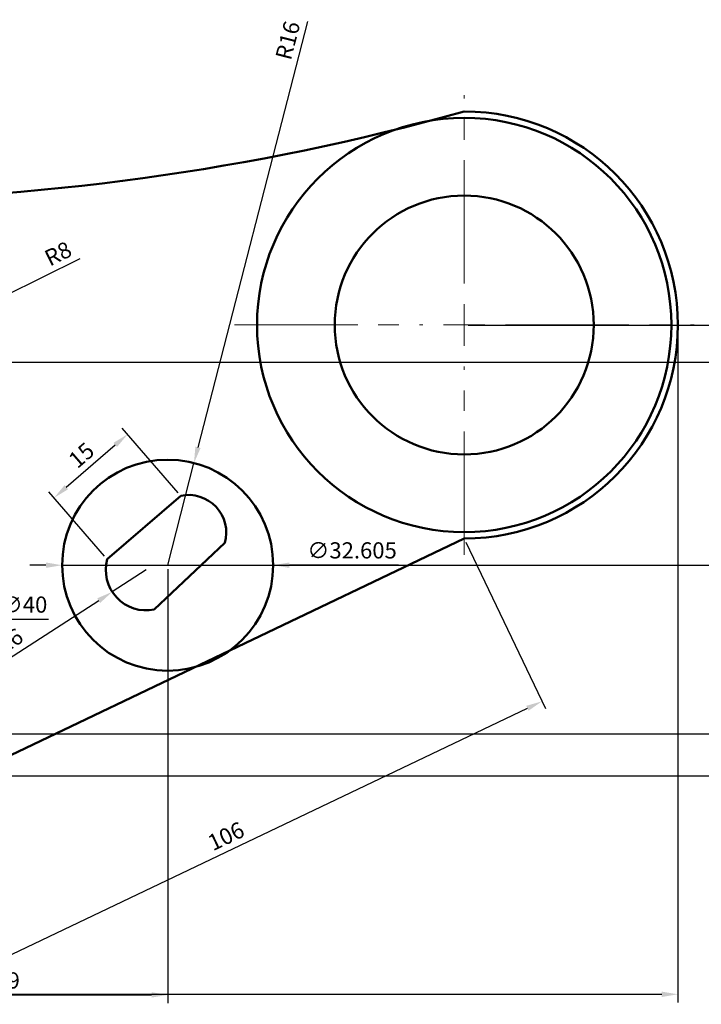
# Model space of a CAD drawing. Units: millimetres. Extents: x 1605 to 2079, y 1280 to 1879.
# Tile 5 of 7: x 1815 to 1920, y 1384 to 1536. Entities that reach past the tile are written whole.
import ezdxf

# ---------------------------------------------------------------- set-up
doc = ezdxf.new("R2010")
doc.units = ezdxf.units.MM
doc.linetypes.add('CENTER2', pattern=[28.575, 19.05, -3.175, 3.175, -3.175])
for name, color, linetype, lineweight in [('M-CNTR', 1, 'CENTER2', 18), ('M-DIMS', 2, 'Continuous', 25), ('M-OUTL', 7, 'Continuous', 50)]:
    doc.layers.add(name, color=color, linetype=linetype, lineweight=lineweight)
doc.styles.get("Standard").update_dxf_attribs({"font": 'arial.ttf'})
doc.dimstyles.new('ISO-25', dxfattribs={"dimtxt": 2.5, "dimasz": 2.5, "dimexe": 1.25, "dimexo": 0.625, "dimtad": 1, "dimdec": 0, "dimtxsty": 'Standard', "dimcen": 2.5, "dimadec": 0, "dimazin": 0, "dimtfac": 1, "dimtdec": 0, "dimtmove": 0, "dimatfit": 3, "dimfxl": 1, "dimarcsym": 0})

# ---------------------------------------------------------------- blocks, each defined once
blk = doc.blocks.new('*U3')
at = {"layer": 'M-CNTR', "color": 0, "transparency": 16777216}
for p, q in [((0, 6.4), (0, 35.5)), ((-35.5, 0), (-6.4, 0)), ((6.4, 0), (35.5, 0)), ((0, -35.5), (0, -6.4))]:
    blk.add_line(p, q, dxfattribs=at)
at = {"layer": 'M-CNTR', "color": 0, "linetype": 'Continuous', "transparency": 16777216}
for p, q in [((0, -3.2), (0, 3.2)), ((-3.2, 0), (3.2, 0))]:
    blk.add_line(p, q, dxfattribs=at)
blk = doc.blocks.new('*D12')
at = {"layer": 'Defpoints', "color": 0, "transparency": 16777216}
for p in [(1650.42, 1488.98), (1916.42, 1488.98), (1916.42, 1385.56)]:
    blk.add_point(p, dxfattribs=at)
at = {"layer": 'M-DIMS', "color": 0, "lineweight": -2, "transparency": 16777216}
for p, q in [((1650.42, 1488.36), (1650.42, 1384.31)), ((1916.42, 1488.36), (1916.42, 1384.31)), ((1652.92, 1385.56), (1913.92, 1385.56))]:
    blk.add_line(p, q, dxfattribs=at)
at = {"layer": 'M-DIMS', "color": 0, "transparency": 16777216}
for points in [[(1652.92, 1385.97), (1652.92, 1385.14), (1650.42, 1385.56)], [(1913.92, 1385.97), (1913.92, 1385.14), (1916.42, 1385.56)]]:
    blk.add_solid(points, dxfattribs=at)
at = {"layer": 'M-DIMS', "color": 0, "transparency": 16777216, "insert": (1783.42, 1387.46), "char_height": 2.5, "attachment_point": 5}
blk.add_mtext('266', dxfattribs=at)
blk = doc.blocks.new('*D18')
at = {"layer": 'Defpoints', "color": 0, "transparency": 16777216}
for p in [(1841.67, 1467.65), (1837.61, 1451.86)]:
    blk.add_point(p, dxfattribs=at)
at = {"layer": 'M-DIMS', "color": 0, "lineweight": -2, "transparency": 16777216}
for p, q in [((1859.21, 1535.89), (1842.29, 1470.07)), ((1837.61, 1451.86), (1841.67, 1467.65))]:
    blk.add_line(p, q, dxfattribs=at)
at = {"layer": 'M-DIMS', "color": 0, "transparency": 16777216}
blk.add_solid([(1841.89, 1470.18), (1842.69, 1469.97), (1841.67, 1467.65)], dxfattribs=at)
at = {"layer": 'M-DIMS', "color": 0, "transparency": 16777216, "insert": (1856.47, 1532.87), "char_height": 2.5, "attachment_point": 5, "rotation": 75.5801}
blk.add_mtext('R16', dxfattribs=at)
blk = doc.blocks.new('*D22')
at = {"layer": 'Defpoints', "color": 0, "transparency": 16777216}
for p in [(1810.14, 1492.31), (1803.42, 1488.98)]:
    blk.add_point(p, dxfattribs=at)
at = {"layer": 'M-DIMS', "color": 0, "lineweight": -2, "transparency": 16777216}
for p, q in [((1824.04, 1499.19), (1812.38, 1493.42)), ((1803.42, 1488.98), (1810.14, 1492.31))]:
    blk.add_line(p, q, dxfattribs=at)
at = {"layer": 'M-DIMS', "color": 0, "transparency": 16777216}
blk.add_solid([(1812.19, 1493.79), (1812.56, 1493.05), (1810.14, 1492.31)], dxfattribs=at)
at = {"layer": 'M-DIMS', "color": 0, "transparency": 16777216, "insert": (1820.82, 1499.72), "char_height": 2.5, "attachment_point": 5, "rotation": 26.3503}
blk.add_mtext('R8', dxfattribs=at)
blk = doc.blocks.new('*D25')
at = {"layer": 'Defpoints', "color": 0, "transparency": 16777216}
for p in [(1883.42, 1455.98), (1895.43, 1430.83), (1787.72, 1410.29)]:
    blk.add_point(p, dxfattribs=at)
at = {"layer": 'M-DIMS', "color": 0, "lineweight": -2, "transparency": 16777216}
for p, q in [((1883.69, 1455.42), (1895.96, 1429.7)), ((1801.99, 1386.22), (1893.17, 1429.75)), ((1787.99, 1409.73), (1800.27, 1384.01))]:
    blk.add_line(p, q, dxfattribs=at)
at = {"layer": 'M-DIMS', "color": 0, "transparency": 16777216}
for points in [[(1892.99, 1430.13), (1893.35, 1429.38), (1895.43, 1430.83)], [(1801.81, 1386.59), (1802.17, 1385.84), (1799.73, 1385.14)]]:
    blk.add_solid(points, dxfattribs=at)
at = {"layer": 'M-DIMS', "color": 0, "transparency": 16777216, "insert": (1846.76, 1409.7), "char_height": 2.5, "attachment_point": 5, "rotation": 25.5234}
blk.add_mtext('106', dxfattribs=at)
blk = doc.blocks.new('*D28')
at = {"layer": 'Defpoints', "color": 0, "transparency": 16777216}
for p in [(1834.3, 1451.14), (1829.05, 1447.75)]:
    blk.add_point(p, dxfattribs=at)
at = {"layer": 'M-DIMS', "color": 0, "lineweight": -2, "transparency": 16777216}
for p, q in [((1834.3, 1451.14), (1829.05, 1447.75)), ((1812.16, 1436.85), (1826.95, 1446.39))]:
    blk.add_line(p, q, dxfattribs=at)
at = {"layer": 'M-DIMS', "color": 0, "transparency": 16777216}
blk.add_solid([(1826.72, 1446.74), (1827.18, 1446.04), (1829.05, 1447.75)], dxfattribs=at)
at = {"layer": 'M-DIMS', "color": 0, "transparency": 16777216, "insert": (1813.35, 1439.88), "char_height": 2.5, "attachment_point": 5, "rotation": 32.8205}
blk.add_mtext('R6', dxfattribs=at)
blk = doc.blocks.new('*D29')
at = {"layer": 'Defpoints', "color": 0, "transparency": 16777216}
for p in [(1831.41, 1472.09), (1839.62, 1462.6), (1828.28, 1452.79)]:
    blk.add_point(p, dxfattribs=at)
at = {"layer": 'M-DIMS', "color": 0, "lineweight": -2, "transparency": 16777216}
for p, q in [((1839.21, 1463.07), (1830.59, 1473.04)), ((1821.95, 1463.91), (1829.51, 1470.45)), ((1827.87, 1453.26), (1819.25, 1463.22))]:
    blk.add_line(p, q, dxfattribs=at)
at = {"layer": 'M-DIMS', "color": 0, "transparency": 16777216}
for points in [[(1829.24, 1470.77), (1829.79, 1470.14), (1831.41, 1472.09)], [(1821.68, 1464.23), (1822.23, 1463.6), (1820.06, 1462.27)]]:
    blk.add_solid(points, dxfattribs=at)
at = {"layer": 'M-DIMS', "color": 0, "transparency": 16777216, "insert": (1824.49, 1468.62), "char_height": 2.5, "attachment_point": 5, "rotation": 40.8746}
blk.add_mtext('15', dxfattribs=at)
blk = doc.blocks.new('*D40')
at = {"layer": 'Defpoints', "color": 0, "transparency": 16777216}
for p in [(1916.42, 1488.98), (1783.42, 1419.31), (2077.9, 1419.31)]:
    blk.add_point(p, dxfattribs=at)
at = {"layer": 'M-DIMS', "color": 0, "lineweight": -2, "transparency": 16777216}
for p, q in [((1917.04, 1488.98), (2079.15, 1488.98)), ((2077.9, 1486.48), (2077.9, 1421.81)), ((1784.04, 1419.31), (2079.15, 1419.31))]:
    blk.add_line(p, q, dxfattribs=at)
at = {"layer": 'M-DIMS', "color": 0, "transparency": 16777216}
for points in [[(2077.48, 1486.48), (2078.32, 1486.48), (2077.9, 1488.98)], [(2077.48, 1421.81), (2078.32, 1421.81), (2077.9, 1419.31)]]:
    blk.add_solid(points, dxfattribs=at)
at = {"layer": 'M-DIMS', "color": 0, "transparency": 16777216, "insert": (2076, 1454.15), "char_height": 2.5, "attachment_point": 5, "rotation": 90}
blk.add_mtext('69.67', dxfattribs=at)
blk = doc.blocks.new('*D43')
at = {"layer": 'Defpoints', "color": 0, "transparency": 16777216}
for p in [(1837.61, 1451.86), (1783.42, 1443.48), (1837.61, 1385.46)]:
    blk.add_point(p, dxfattribs=at)
at = {"layer": 'M-DIMS', "color": 0, "lineweight": -2, "transparency": 16777216}
for p, q in [((1837.61, 1451.24), (1837.61, 1384.21)), ((1783.42, 1442.85), (1783.42, 1384.21)), ((1785.92, 1385.46), (1835.11, 1385.46))]:
    blk.add_line(p, q, dxfattribs=at)
at = {"layer": 'M-DIMS', "color": 0, "transparency": 16777216}
for points in [[(1785.92, 1385.88), (1785.92, 1385.05), (1783.42, 1385.46)], [(1835.11, 1385.88), (1835.11, 1385.05), (1837.61, 1385.46)]]:
    blk.add_solid(points, dxfattribs=at)
at = {"layer": 'M-DIMS', "color": 0, "transparency": 16777216, "insert": (1810.51, 1387.37), "char_height": 2.5, "attachment_point": 5}
blk.add_mtext('54.19', dxfattribs=at)
blk = doc.blocks.new('*D46')
at = {"layer": 'Defpoints', "color": 0, "transparency": 16777216}
for p in [(1883.42, 1488.98), (2077.9, 1488.98), (1837.61, 1451.86)]:
    blk.add_point(p, dxfattribs=at)
at = {"layer": 'M-DIMS', "color": 0, "lineweight": -2, "transparency": 16777216}
for p, q in [((1884.04, 1488.98), (2079.15, 1488.98)), ((2077.9, 1454.36), (2077.9, 1486.48)), ((1838.23, 1451.86), (2079.15, 1451.86))]:
    blk.add_line(p, q, dxfattribs=at)
at = {"layer": 'M-DIMS', "color": 0, "transparency": 16777216}
for points in [[(2077.48, 1486.48), (2078.32, 1486.48), (2077.9, 1488.98)], [(2077.48, 1454.36), (2078.32, 1454.36), (2077.9, 1451.86)]]:
    blk.add_solid(points, dxfattribs=at)
at = {"layer": 'M-DIMS', "color": 0, "transparency": 16777216, "insert": (2076, 1470.42), "char_height": 2.5, "attachment_point": 5, "rotation": 90}
blk.add_mtext('37.12', dxfattribs=at)
blk = doc.blocks.new('*D51')
at = {"layer": 'Defpoints', "color": 0, "transparency": 16777216}
for p in [(1624.07, 1483.2), (1984.76, 1483.2), (1947.57, 1425.73)]:
    blk.add_point(p, dxfattribs=at)
at = {"layer": 'M-DIMS', "color": 0, "lineweight": -2, "transparency": 16777216}
for p, q in [((1984.13, 1483.2), (1622.82, 1483.2)), ((1624.07, 1428.23), (1624.07, 1480.7)), ((1946.94, 1425.73), (1622.82, 1425.73))]:
    blk.add_line(p, q, dxfattribs=at)
at = {"layer": 'M-DIMS', "color": 0, "transparency": 16777216}
for points in [[(1623.65, 1480.7), (1624.48, 1480.7), (1624.07, 1483.2)], [(1623.65, 1428.23), (1624.48, 1428.23), (1624.07, 1425.73)]]:
    blk.add_solid(points, dxfattribs=at)
at = {"layer": 'M-DIMS', "color": 0, "transparency": 16777216, "insert": (1622.17, 1454.47), "char_height": 2.5, "attachment_point": 5, "rotation": 90}
blk.add_mtext('57.47', dxfattribs=at)
blk = doc.blocks.new('*D64')
at = {"layer": 'Defpoints', "color": 0, "transparency": 16777216}
for p in [(1763.42, 1443.48), (1803.42, 1443.48)]:
    blk.add_point(p, dxfattribs=at)
at = {"layer": 'M-DIMS', "color": 0, "lineweight": -2, "transparency": 16777216}
for p, q in [((1760.92, 1443.48), (1758.42, 1443.48)), ((1763.42, 1443.48), (1803.42, 1443.48)), ((1819.19, 1443.48), (1805.92, 1443.48))]:
    blk.add_line(p, q, dxfattribs=at)
at = {"layer": 'M-DIMS', "color": 0, "transparency": 16777216}
for points in [[(1760.92, 1443.9), (1760.92, 1443.06), (1763.42, 1443.48)], [(1805.92, 1443.9), (1805.92, 1443.06), (1803.42, 1443.48)]]:
    blk.add_solid(points, dxfattribs=at)
at = {"layer": 'M-DIMS', "color": 0, "transparency": 16777216, "insert": (1815.42, 1445.45), "char_height": 2.5, "attachment_point": 5, "rotation": 359.9999}
blk.add_mtext('∅40', dxfattribs=at)
blk = doc.blocks.new('*D67')
at = {"layer": 'Defpoints', "color": 0, "transparency": 16777216}
for p in [(1821.3, 1451.86), (1853.91, 1451.86)]:
    blk.add_point(p, dxfattribs=at)
at = {"layer": 'M-DIMS', "color": 0, "lineweight": -2, "transparency": 16777216}
for p, q in [((1818.8, 1451.86), (1816.3, 1451.86)), ((1821.3, 1451.86), (1853.91, 1451.86)), ((1873.28, 1451.86), (1856.41, 1451.86))]:
    blk.add_line(p, q, dxfattribs=at)
at = {"layer": 'M-DIMS', "color": 0, "transparency": 16777216}
for points in [[(1818.8, 1452.28), (1818.8, 1451.45), (1821.3, 1451.86)], [(1856.41, 1452.28), (1856.41, 1451.45), (1853.91, 1451.86)]]:
    blk.add_solid(points, dxfattribs=at)
at = {"layer": 'M-DIMS', "color": 0, "transparency": 16777216, "insert": (1866.09, 1453.83), "char_height": 2.5, "attachment_point": 5, "rotation": 359.9995}
blk.add_mtext('∅32.605', dxfattribs=at)

msp = doc.modelspace()

# ---------------------------------------------------------------- linework, layer by layer
at = {"layer": 'M-OUTL'}
for p, q in [((1828.2752, 1452.7862), (1839.6174, 1462.6023)), ((1787.7246, 1410.2904), (1883.4159, 1455.9806)), ((1846.4454, 1455.2963), (1835.5316, 1445.006))]:
    msp.add_line(p, q, dxfattribs=at)
for centre, radius in [((1883.4159, 1488.9806), 32), ((1883.4159, 1488.9806), 20), ((1837.6066, 1451.8622), 16.3026)]:
    msp.add_circle(centre, radius, dxfattribs=at)
for centre, radius, start, end in [((1783.4159, 1878.8069), 370.5739, 254.344556, 285.655444), ((1883.4159, 1488.9806), 33, 270, 90), ((1840.8061, 1456.8696), 5.8547, 344.411098, 101.714746), ((1834.3044, 1451.1354), 6.2511, 164.687519, 281.322073)]:
    msp.add_arc(centre, radius, start, end, dxfattribs=at)

# ---------------------------------------------------------------- block references
at = {"layer": 'M-CNTR'}
msp.add_blockref('*U3', (1883.4159, 1488.9806), dxfattribs=at)

# ---------------------------------------------------------------- dimensions: what is measured, and where the dimension line sits
at = {"layer": 'M-DIMS'}
for center, mpoint, picture, middle in [((1837.6066, 1451.8622), (1841.6664, 1467.6512), '*D18', (1858.3134, 1532.3936)), ((1803.4159, 1488.9806), (1810.1366, 1492.3095), '*D22', (1821.6668, 1498.0207)), ((1834.3044, 1451.1354), (1829.0511, 1447.7473), '*D28', (1814.3783, 1438.2839))]:
    dim = msp.add_radius_dim(center=center, mpoint=mpoint, dimstyle='ISO-25', override={"dimclrd": 0, "dimclre": 0, "dimclrt": 0}, dxfattribs=at)
    dim.commit()
    dim.dimension.update_dxf_attribs({"geometry": picture, "text_midpoint": middle, "dimtype": 164})
for base, p1, p2, override, picture, middle in [((1916.4159, 1385.5558), (1650.4159, 1488.9806), (1916.4159, 1488.9806), {"dimclrd": 0, "dimclre": 0, "dimclrt": 0}, '*D12', (1783.4159, 1387.4572)), ((1837.6066, 1385.4644), (1783.4159, 1443.479), (1837.6066, 1451.8622), {"dimdec": 2, "dimlfac": 1, "dimrnd": 0, "dimzin": 0, "dimdsep": 46, "dimlunit": 2}, '*D43', (1810.5112, 1387.3659))]:
    dim = msp.add_linear_dim(base=base, p1=p1, p2=p2, dimstyle='ISO-25', override=override, dxfattribs=at)
    dim.commit()
    dim.dimension.update_dxf_attribs({"geometry": picture, "text_midpoint": middle})
for base, p1, p2, picture, middle in [((2077.8984, 1419.3145), (1916.4159, 1488.9806), (1783.4159, 1419.3145), '*D40', (2075.997, 1454.1475)), ((2077.8984, 1488.9806), (1837.6066, 1451.8622), (1883.4159, 1488.9806), '*D46', (2075.9961, 1470.4214)), ((1624.0659, 1483.2046), (1947.5688, 1425.7344), (1984.7564, 1483.2046), '*D51', (1622.1695, 1454.4695))]:
    dim = msp.add_linear_dim(base=base, p1=p1, p2=p2, angle=90, dimstyle='ISO-25', override={"dimdec": 2, "dimlfac": 1, "dimrnd": 0, "dimzin": 0, "dimdsep": 46, "dimlunit": 2}, dxfattribs=at)
    dim.commit()
    dim.dimension.update_dxf_attribs({"geometry": picture, "text_midpoint": middle})
for p1, p2, distance, picture, middle in [((1828.2752, 1452.7862), (1839.6174, 1462.6023), 12.5488, '*D29', (1824.49, 1468.6207)), ((1787.7246, 1410.2904), (1883.4159, 1455.9806), -27.8723, '*D25', (1846.7605, 1409.6992))]:
    dim = msp.add_aligned_dim(p1=p1, p2=p2, distance=distance, dimstyle='ISO-25', override={"dimclrd": 0, "dimclre": 0, "dimclrt": 0}, dxfattribs=at)
    dim.commit()
    dim.dimension.update_dxf_attribs({"geometry": picture, "text_midpoint": middle})
dim = msp.add_diameter_dim_2p(p1=(1821.304, 1451.8623), p2=(1853.9092, 1451.862), dimstyle='ISO-25', override={"dimdec": 3, "dimlfac": 1, "dimrnd": 0, "dimzin": 0, "dimdsep": 46, "dimlunit": 2}, dxfattribs=at)
dim.commit()
dim.dimension.update_dxf_attribs({"geometry": '*D67', "text_midpoint": (1866.0929, 1451.8619)})
dim = msp.add_diameter_dim_2p(p1=(1763.4159, 1443.479), p2=(1803.4159, 1443.479), dimstyle='ISO-25', override={"dimdec": 0, "dimlfac": 1, "dimrnd": 0, "dimzin": 0, "dimdsep": 46, "dimlunit": 2}, dxfattribs=at)
dim.commit()
dim.dimension.update_dxf_attribs({"geometry": '*D64', "text_midpoint": (1815.4159, 1443.479), "dimtype": 163})

doc.saveas('drawing.dxf')
